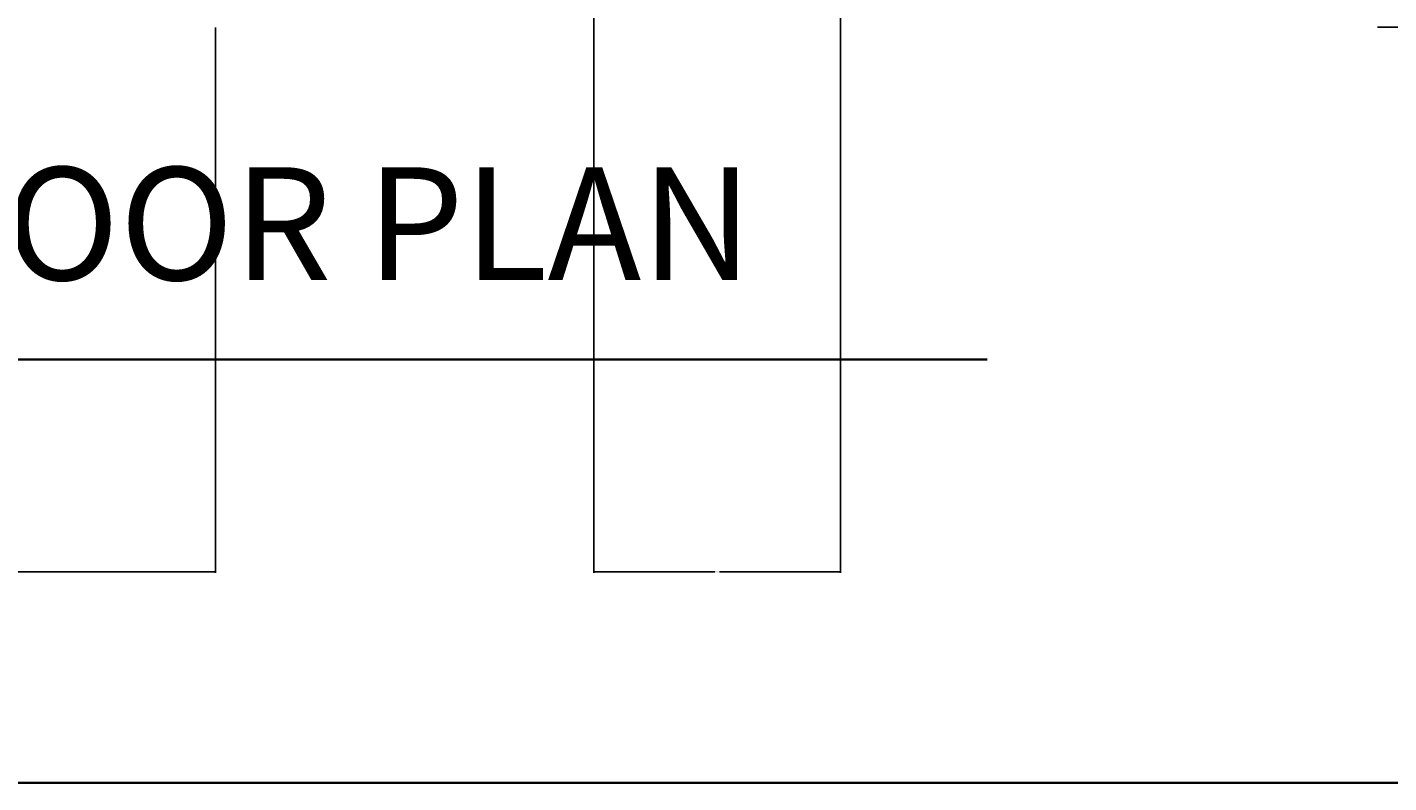
# Model space of a CAD drawing. Units: inches. Extents: x 2310 to 2937, y 1113 to 2410.
# Tile 9 of 23: x 2609 to 2826, y 1616 to 1737. Entities that reach past the tile are written whole.
import ezdxf

# ---------------------------------------------------------------- set-up
doc = ezdxf.new("R2010")
doc.units = ezdxf.units.IN
doc.layers.add('A-ANNO-DIMS', color=2, linetype='Continuous', lineweight=18)
doc.layers.add('A-ANNO-TTLB', color=7, linetype='Continuous', lineweight=35)
doc.styles.get("Standard").update_dxf_attribs({"font": 'arial.ttf'})
doc.dimstyles.get("Standard").update_dxf_attribs({"dimtxt": 0.18, "dimasz": 0.18, "dimexe": 0.18, "dimexo": 0.0625, "dimgap": 0.09, "dimtad": 0, "dimtih": 1, "dimtoh": 1, "dimdec": 4, "dimzin": 0, "dimdsep": 46, "dimtxsty": 'Standard', "dimcen": 0.09, "dimadec": 0, "dimazin": 0, "dimtfac": 1, "dimtdec": 4, "dimtofl": 0, "dimtmove": 0, "dimatfit": 3, "dimfxl": 1, "dimtolj": 1, "dimtzin": 0, "dimarcsym": 0})

# ---------------------------------------------------------------- blocks, each defined once
blk = doc.blocks.new('*D42')
at = {"layer": 'A-ANNO-DIMS', "color": 0, "lineweight": -2, "transparency": 16777216}
for p, q in [((2699.14, 2347.45), (2699.14, 1649.5)), ((2738.49, 2347.45), (2738.49, 1649.5)), ((2699.32, 1649.68), (2718.42, 1649.68)), ((2738.31, 1649.68), (2719.21, 1649.68))]:
    blk.add_line(p, q, dxfattribs=at)
at = {"layer": 'A-ANNO-DIMS', "color": 0, "transparency": 16777216}
for points in [[(2699.32, 1649.71), (2699.32, 1649.65), (2699.14, 1649.68)], [(2738.31, 1649.71), (2738.31, 1649.65), (2738.49, 1649.68)]]:
    blk.add_solid(points, dxfattribs=at)
at = {"layer": 'Defpoints', "color": 0, "transparency": 16777216}
for p in [(2699.14, 2347.51), (2738.49, 2347.51), (2738.49, 1649.68)]:
    blk.add_point(p, dxfattribs=at)
at = {"layer": 'A-ANNO-DIMS', "color": 0, "transparency": 16777216, "insert": (2718.81, 1649.68), "char_height": 0.18, "attachment_point": 5}
blk.add_mtext('\\A1;39.35', dxfattribs=at)
blk = doc.blocks.new('*D44')
at = {"layer": 'A-ANNO-DIMS', "color": 0, "lineweight": -2, "transparency": 16777216}
for p, q in [((2558.31, 1736.45), (2558.31, 1649.5)), ((2638.89, 1736.45), (2638.89, 1649.5)), ((2558.49, 1649.68), (2598.21, 1649.68)), ((2638.71, 1649.68), (2598.99, 1649.68))]:
    blk.add_line(p, q, dxfattribs=at)
at = {"layer": 'A-ANNO-DIMS', "color": 0, "transparency": 16777216}
for points in [[(2558.49, 1649.71), (2558.49, 1649.65), (2558.31, 1649.68)], [(2638.71, 1649.71), (2638.71, 1649.65), (2638.89, 1649.68)]]:
    blk.add_solid(points, dxfattribs=at)
at = {"layer": 'Defpoints', "color": 0, "transparency": 16777216}
for p in [(2558.31, 1736.51), (2638.89, 1736.51), (2638.89, 1649.68)]:
    blk.add_point(p, dxfattribs=at)
at = {"layer": 'A-ANNO-DIMS', "color": 0, "transparency": 16777216, "insert": (2598.6, 1649.68), "char_height": 0.18, "attachment_point": 5}
blk.add_mtext('\\A1;80.59', dxfattribs=at)
blk = doc.blocks.new('*D45')
at = {"layer": 'A-ANNO-DIMS', "color": 0, "lineweight": -2, "transparency": 16777216}
for p, q in [((2824.05, 1759.67), (2858.02, 1759.67)), ((2857.84, 1759.49), (2857.84, 1748.27)), ((2857.84, 1736.69), (2857.84, 1747.91)), ((2824.05, 1736.51), (2858.02, 1736.51))]:
    blk.add_line(p, q, dxfattribs=at)
at = {"layer": 'A-ANNO-DIMS', "color": 0, "transparency": 16777216}
for points in [[(2857.81, 1759.49), (2857.87, 1759.49), (2857.84, 1759.67)], [(2857.81, 1736.69), (2857.87, 1736.69), (2857.84, 1736.51)]]:
    blk.add_solid(points, dxfattribs=at)
at = {"layer": 'Defpoints', "color": 0, "transparency": 16777216}
for p in [(2823.99, 1759.67), (2857.84, 1759.67), (2823.99, 1736.51)]:
    blk.add_point(p, dxfattribs=at)
at = {"layer": 'A-ANNO-DIMS', "color": 0, "transparency": 16777216, "insert": (2857.84, 1748.09), "char_height": 0.18, "attachment_point": 5}
blk.add_mtext('\\A1;23.154', dxfattribs=at)

msp = doc.modelspace()

# ---------------------------------------------------------------- linework, layer by layer
at = {"layer": 'A-ANNO-TTLB'}
msp.add_line((2487.6418, 1683.5307), (2761.8399, 1683.5307), dxfattribs=at)
msp.add_lwpolyline([(2310.2498, 2409.8427), (2937.0534, 2409.8427), (2937.0534, 1616.036), (2310.2498, 1616.036)], close=True, dxfattribs=at)

# ---------------------------------------------------------------- texts
at = {"layer": 'A-ANNO-TTLB', "insert": (2507.293, 1714.1887), "char_height": 18, "attachment_point": 1}
msp.add_mtext_dynamic_manual_height_columns('FIRST FLOOR PLAN', width=651.219844, gutter_width=12.5, heights=[0], dxfattribs=at)

# ---------------------------------------------------------------- dimensions: what is measured, and where the dimension line sits
at = {"layer": 'A-ANNO-DIMS'}
for base, p1, p2, picture, middle in [((2738.4859, 1649.6807), (2699.1394, 2347.5139), (2738.4859, 2347.5139), '*D42', (2718.8127, 1649.6807)), ((2638.8921, 1649.6807), (2558.3065, 1736.5139), (2638.8921, 1736.5139), '*D44', (2598.5993, 1649.6807))]:
    dim = msp.add_linear_dim(base=base, p1=p1, p2=p2, dimstyle='Standard', override={"dimdec": 2, "dimlfac": 1, "dimrnd": 0, "dimzin": 0, "dimdsep": 46, "dimlunit": 2}, dxfattribs=at)
    dim.commit()
    dim.dimension.update_dxf_attribs({"geometry": picture, "text_midpoint": middle})
dim = msp.add_linear_dim(base=(2857.83594, 1759.66842), p1=(2823.98594, 1736.51394), p2=(2823.98594, 1759.66842), angle=90, dimstyle='Standard', override={"dimdec": 3, "dimlfac": 1, "dimrnd": 0, "dimzin": 0, "dimdsep": 46, "dimlunit": 2}, dxfattribs=at)
dim.commit()
dim.dimension.update_dxf_attribs({"geometry": '*D45', "text_midpoint": (2857.83594, 1748.09118)})

doc.saveas('drawing.dxf')
